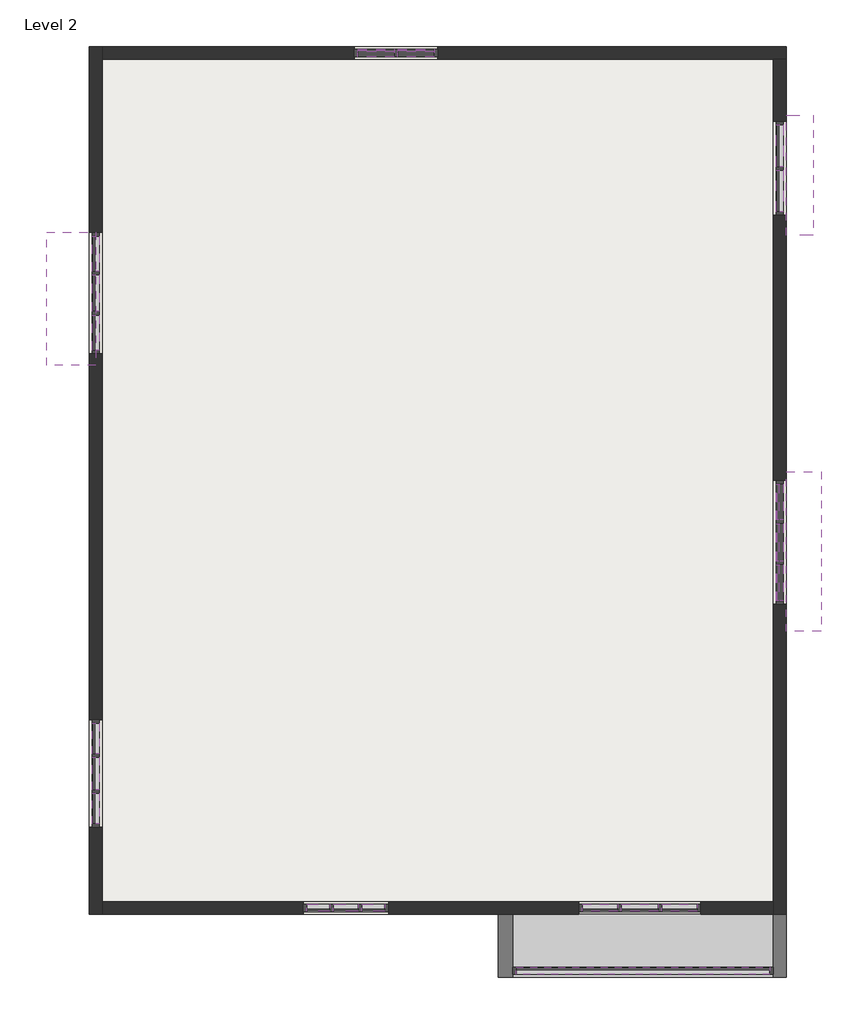
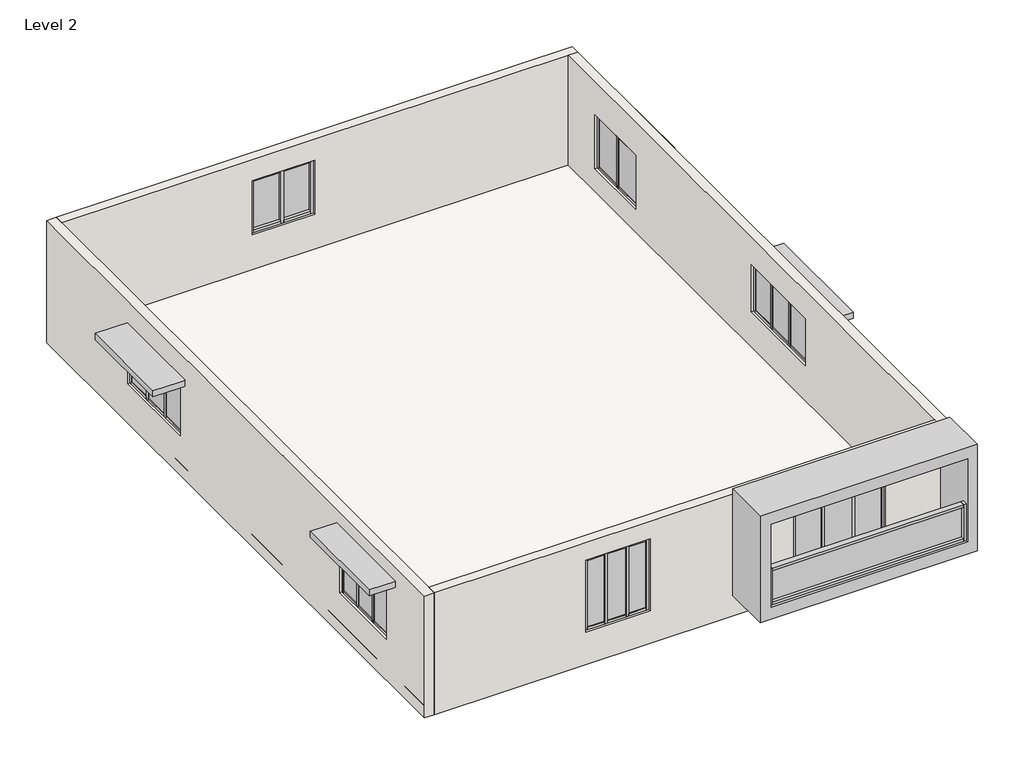
# One storey: 68 members, 20 plates, 4 proxies, 4 walls, 1 roof.
"""IFC4 building model written with IfcOpenShell, lengths in millimetres."""

from ifc_helpers import new_model, si_unit, frame, origin, place, context, project, spatial, polyline, outline, extrude, faceted_brep, transform, mapped, element, save
from components import generic_models_10_generic_models_10_e59920a7, generic_models_13_generic_models_13_81a3a1d9, generic_models_4_generic_models_4_7a9117e9, generic_models_9_generic_models_9_c0a8784b, member_bc7dbe04, member_dc106669, member_3fd415ec, member_f80a073c, member_00d99baf, member_d3852687, member_f51f5eff, member_1cdc6c9a, member_1d73318e, member_ea77439e, member_3a0a7659, member_051277f3, member_afffad75, member_dad99500, member_d9f78736, member_05f3a264, member_d4123ca4, member_668e8779, member_8c893cff, member_c9631cd1, member_eeb7212f, member_0bb20091, member_43a8b99b, member_a81ad59a, member_ef5723a8, member_5215b92c, member_553ffa17, member_c0163ebe, system_panel_glazed_42f26034, system_panel_glazed_4ea5c58e, system_panel_glazed_209adb3c, system_panel_glazed_df754354, system_panel_glazed_4996dcf2, system_panel_glazed_4f773535, system_panel_glazed_f0f913a6, system_panel_glazed_204414d1, system_panel_glazed_c810d226, system_panel_glazed_a6da17b0, system_panel_glazed_9e0010b7, system_panel_glazed_2a0e46e6, system_panel_glazed_327d625d

model = new_model("IFC4")

# Units and contexts
model_context = context("Model", 3, world=origin())
ifc_project = project(units=[si_unit("LENGTHUNIT", "METRE", prefix="MILLI")], contexts=[model_context])

# Site, building, storey
site = spatial("IfcSite", under=ifc_project)
building = spatial("IfcBuilding", under=site)
storey = spatial("IfcBuildingStorey", under=building, Name="Level 2", Elevation=3048.0)

# Proxies
placement = place(None, origin())
generic_models_10_generic_models_10_shape = generic_models_10_generic_models_10_e59920a7(model_context)
element("IfcBuildingElementProxy", 1, Name="Generic Models 10 : Generic Models 10", ObjectType="Generic Models 10 : Generic Models 10", at=placement, inside=storey, context=model_context, shape_type="MappedRepresentation", body=[
    mapped(generic_models_10_generic_models_10_shape, transform((0.0, 0.0, 0.0), x_axis=(1.0, 0.0, 0.0), y_axis=(0.0, 1.0, 0.0), z_axis=(0.0, 0.0, 1.0))),
])
generic_models_13_generic_models_13_shape = generic_models_13_generic_models_13_81a3a1d9(model_context)
element("IfcBuildingElementProxy", 2, Name="Generic Models 13 : Generic Models 13", ObjectType="Generic Models 13 : Generic Models 13", at=placement, inside=storey, context=model_context, shape_type="MappedRepresentation", body=[
    mapped(generic_models_13_generic_models_13_shape, transform((0.0, 0.0, 0.0), x_axis=(1.0, 0.0, 0.0), y_axis=(0.0, 1.0, 0.0), z_axis=(0.0, 0.0, 1.0))),
])
generic_models_4_generic_models_4_shape = generic_models_4_generic_models_4_7a9117e9(model_context)
element("IfcBuildingElementProxy", 3, Name="Generic Models 4 : Generic Models 4", ObjectType="Generic Models 4 : Generic Models 4", at=placement, inside=storey, context=model_context, shape_type="MappedRepresentation", body=[
    mapped(generic_models_4_generic_models_4_shape, transform((0.0, 0.0, 0.0), x_axis=(1.0, 0.0, 0.0), y_axis=(0.0, 1.0, 0.0), z_axis=(0.0, 0.0, 1.0))),
])
generic_models_9_generic_models_9_shape = generic_models_9_generic_models_9_c0a8784b(model_context)
element("IfcBuildingElementProxy", 4, Name="Generic Models 9 : Generic Models 9", ObjectType="Generic Models 9 : Generic Models 9", at=placement, inside=storey, context=model_context, shape_type="MappedRepresentation", body=[
    mapped(generic_models_9_generic_models_9_shape, transform((0.0, 0.0, 0.0), x_axis=(1.0, 0.0, 0.0), y_axis=(0.0, 1.0, 0.0), z_axis=(0.0, 0.0, 1.0))),
])

# Members
member_shape = member_bc7dbe04(model_context)
element("IfcMember", 5, ObjectType="Rectangular Mullion : 2.5\" x 5\" rectangular", at=placement, inside=storey, context=model_context, shape_type="MappedRepresentation", body=[
    mapped(member_shape, transform((-11428.8359258, -11686.7777232, 3860.2469154), x_axis=(0.0, 0.0, -1.0), y_axis=(0.0, 1.0, 0.0), z_axis=(1.0, 0.0, 0.0))),
])
member_2_shape = member_dc106669(model_context)
element("IfcMember", 6, ObjectType="Rectangular Mullion : 2.5\" x 5\" rectangular", at=placement, inside=storey, context=model_context, shape_type="MappedRepresentation", body=[
    mapped(member_2_shape, transform((-11936.8359258, -11686.7777232, 3860.2469154), x_axis=(0.0, 0.0, -1.0), y_axis=(0.0, 1.0, 0.0), z_axis=(1.0, 0.0, 0.0))),
])
element("IfcMember", 7, ObjectType="Rectangular Mullion : 2.5\" x 5\" rectangular", at=placement, inside=storey, context=model_context, shape_type="MappedRepresentation", body=[
    mapped(member_2_shape, transform((-10952.5859258, -11686.7777232, 3860.2469154), x_axis=(0.0, 0.0, -1.0), y_axis=(0.0, 1.0, 0.0), z_axis=(1.0, 0.0, 0.0))),
])
element("IfcMember", 8, ObjectType="Rectangular Mullion : 2.5\" x 5\" rectangular", at=placement, inside=storey, context=model_context, shape_type="MappedRepresentation", body=[
    mapped(member_2_shape, transform((-11365.3359258, -11686.7777232, 5656.7140305), x_axis=(0.0, 0.0, 1.0), y_axis=(0.0, 1.0, 0.0), z_axis=(-1.0, 0.0, 0.0))),
])
element("IfcMember", 9, ObjectType="Rectangular Mullion : 2.5\" x 5\" rectangular", at=placement, inside=storey, context=model_context, shape_type="MappedRepresentation", body=[
    mapped(member_2_shape, transform((-12349.5859258, -11686.7777232, 5656.7140305), x_axis=(0.0, 0.0, 1.0), y_axis=(0.0, 1.0, 0.0), z_axis=(-1.0, 0.0, 0.0))),
])
element("IfcMember", 10, ObjectType="Rectangular Mullion : 2.5\" x 5\" rectangular", at=placement, inside=storey, context=model_context, shape_type="MappedRepresentation", body=[
    mapped(member_shape, transform((-11873.3359258, -11686.7777232, 5656.7140305), x_axis=(0.0, 0.0, 1.0), y_axis=(0.0, 1.0, 0.0), z_axis=(-1.0, 0.0, 0.0))),
])
member_3_shape = member_3fd415ec(model_context)
element("IfcMember", 11, ObjectType="Rectangular Mullion : 2.5\" x 5\" rectangular", at=placement, inside=storey, context=model_context, shape_type="MappedRepresentation", body=[
    mapped(member_3_shape, transform((-11905.0859258, -11686.7777232, 3860.2469154), x_axis=(-1.0, 0.0, 0.0), y_axis=(0.0, 1.0, 0.0), z_axis=(0.0, 0.0, -1.0))),
])
element("IfcMember", 12, ObjectType="Rectangular Mullion : 2.5\" x 5\" rectangular", at=placement, inside=storey, context=model_context, shape_type="MappedRepresentation", body=[
    mapped(member_3_shape, transform((-11397.0859258, -11686.7777232, 3860.2469154), x_axis=(-1.0, 0.0, 0.0), y_axis=(0.0, 1.0, 0.0), z_axis=(0.0, 0.0, -1.0))),
])
member_4_shape = member_f80a073c(model_context)
element("IfcMember", 13, ObjectType="Rectangular Mullion : 2.5\" x 5\" rectangular", at=placement, inside=storey, context=model_context, shape_type="MappedRepresentation", body=[
    mapped(member_4_shape, transform((-12413.0859258, -11686.7777232, 3860.2469154), x_axis=(-1.0, 0.0, 0.0), y_axis=(0.0, 1.0, 0.0), z_axis=(0.0, 0.0, -1.0))),
])
element("IfcMember", 14, ObjectType="Rectangular Mullion : 2.5\" x 5\" rectangular", at=placement, inside=storey, context=model_context, shape_type="MappedRepresentation", body=[
    mapped(member_4_shape, transform((-10889.0859258, -11686.7777232, 5656.7140305), x_axis=(1.0, 0.0, 0.0), y_axis=(0.0, 1.0, 0.0), z_axis=(0.0, 0.0, 1.0))),
])
member_5_shape = member_00d99baf(model_context)
element("IfcMember", 15, ObjectType="Rectangular Mullion : 2.5\" x 5\" rectangular", at=placement, inside=storey, context=model_context, shape_type="MappedRepresentation", body=[
    mapped(member_5_shape, transform((-6018.6359258, -11686.7777232, 5933.9332237), x_axis=(0.0, 0.0, 1.0), y_axis=(0.0, 1.0, 0.0), z_axis=(-1.0, 0.0, 0.0))),
])
element("IfcMember", 16, ObjectType="Rectangular Mullion : 2.5\" x 5\" rectangular", at=placement, inside=storey, context=model_context, shape_type="MappedRepresentation", body=[
    mapped(member_5_shape, transform((-7434.6859258, -11686.7777232, 5933.9332237), x_axis=(0.0, 0.0, 1.0), y_axis=(0.0, 1.0, 0.0), z_axis=(-1.0, 0.0, 0.0))),
])
member_6_shape = member_d3852687(model_context)
element("IfcMember", 17, ObjectType="Rectangular Mullion : 2.5\" x 5\" rectangular", at=placement, inside=storey, context=model_context, shape_type="MappedRepresentation", body=[
    mapped(member_6_shape, transform((-6742.5359258, -11686.7777232, 5933.9332237), x_axis=(0.0, 0.0, 1.0), y_axis=(0.0, 1.0, 0.0), z_axis=(-1.0, 0.0, 0.0))),
])
element("IfcMember", 18, ObjectType="Rectangular Mullion : 2.5\" x 5\" rectangular", at=placement, inside=storey, context=model_context, shape_type="MappedRepresentation", body=[
    mapped(member_6_shape, transform((-6082.1359258, -11686.7777232, 3853.2485641), x_axis=(0.0, 0.0, -1.0), y_axis=(0.0, 1.0, 0.0), z_axis=(1.0, 0.0, 0.0))),
])
element("IfcMember", 19, ObjectType="Rectangular Mullion : 2.5\" x 5\" rectangular", at=placement, inside=storey, context=model_context, shape_type="MappedRepresentation", body=[
    mapped(member_5_shape, transform((-6806.0359258, -11686.7777232, 3853.2485641), x_axis=(0.0, 0.0, -1.0), y_axis=(0.0, 1.0, 0.0), z_axis=(1.0, 0.0, 0.0))),
])
element("IfcMember", 20, ObjectType="Rectangular Mullion : 2.5\" x 5\" rectangular", at=placement, inside=storey, context=model_context, shape_type="MappedRepresentation", body=[
    mapped(member_5_shape, transform((-5389.9859258, -11686.7777232, 3853.2485641), x_axis=(0.0, 0.0, -1.0), y_axis=(0.0, 1.0, 0.0), z_axis=(1.0, 0.0, 0.0))),
])
member_7_shape = member_f51f5eff(model_context)
element("IfcMember", 21, ObjectType="Rectangular Mullion : 2.5\" x 5\" rectangular", at=placement, inside=storey, context=model_context, shape_type="MappedRepresentation", body=[
    mapped(member_7_shape, transform((-6774.2859258, -11686.7777232, 3853.2485641), x_axis=(-1.0, 0.0, 0.0), y_axis=(0.0, 1.0, 0.0), z_axis=(0.0, 0.0, -1.0))),
])
element("IfcMember", 22, ObjectType="Rectangular Mullion : 2.5\" x 5\" rectangular", at=placement, inside=storey, context=model_context, shape_type="MappedRepresentation", body=[
    mapped(member_7_shape, transform((-6050.3859258, -11686.7777232, 3853.2485641), x_axis=(-1.0, 0.0, 0.0), y_axis=(0.0, 1.0, 0.0), z_axis=(0.0, 0.0, -1.0))),
])
member_8_shape = member_1cdc6c9a(model_context)
element("IfcMember", 23, ObjectType="Rectangular Mullion : 2.5\" x 5\" rectangular", at=placement, inside=storey, context=model_context, shape_type="MappedRepresentation", body=[
    mapped(member_8_shape, transform((-7498.1859258, -11686.7777232, 3853.2485641), x_axis=(-1.0, 0.0, 0.0), y_axis=(0.0, 1.0, 0.0), z_axis=(0.0, 0.0, -1.0))),
])
element("IfcMember", 24, ObjectType="Rectangular Mullion : 2.5\" x 5\" rectangular", at=placement, inside=storey, context=model_context, shape_type="MappedRepresentation", body=[
    mapped(member_8_shape, transform((-5326.4859258, -11686.7777232, 5933.9332237), x_axis=(1.0, 0.0, 0.0), y_axis=(0.0, 1.0, 0.0), z_axis=(0.0, 0.0, 1.0))),
])
member_9_shape = member_1d73318e(model_context)
element("IfcMember", 25, ObjectType="Rectangular Mullion : 2.5\" x 5\" rectangular", at=placement, inside=storey, context=model_context, shape_type="MappedRepresentation", body=[
    mapped(member_9_shape, transform((-8679.2859258, -12804.3777232, 4777.3649741), x_axis=(-1.0, 0.0, 0.0), y_axis=(0.0, -1.0, 0.0), z_axis=(0.0, 0.0, 1.0))),
])
member_10_shape = member_ea77439e(model_context)
element("IfcMember", 26, ObjectType="Rectangular Mullion : 2.5\" x 5\" rectangular", at=placement, inside=storey, context=model_context, shape_type="MappedRepresentation", body=[
    mapped(member_10_shape, transform((-4094.5859258, -12804.3777232, 4777.3649741), x_axis=(0.0, 0.0, 1.0), y_axis=(0.0, -1.0, 0.0), z_axis=(1.0, 0.0, 0.0))),
])
element("IfcMember", 27, ObjectType="Rectangular Mullion : 2.5\" x 5\" rectangular", at=placement, inside=storey, context=model_context, shape_type="MappedRepresentation", body=[
    mapped(member_10_shape, transform((-8615.7859258, -12804.3777232, 3860.2469154), x_axis=(0.0, 0.0, -1.0), y_axis=(0.0, -1.0, 0.0), z_axis=(-1.0, 0.0, 0.0))),
])
element("IfcMember", 28, ObjectType="Rectangular Mullion : 2.5\" x 5\" rectangular", at=placement, inside=storey, context=model_context, shape_type="MappedRepresentation", body=[
    mapped(member_9_shape, transform((-4031.0859258, -12804.3777232, 3860.2469154), x_axis=(1.0, 0.0, 0.0), y_axis=(0.0, -1.0, 0.0), z_axis=(0.0, 0.0, -1.0))),
])
member_11_shape = member_3a0a7659(model_context)
element("IfcMember", 29, ObjectType="Rectangular Mullion : 2.5\" x 5\" rectangular", at=placement, inside=storey, context=model_context, shape_type="MappedRepresentation", body=[
    mapped(member_11_shape, transform((-3916.7859258, 1527.5722768, 3931.1298826), x_axis=(0.0, 0.0, -1.0), y_axis=(1.0, 0.0, 0.0), z_axis=(0.0, -1.0, 0.0))),
])
element("IfcMember", 30, ObjectType="Rectangular Mullion : 2.5\" x 5\" rectangular", at=placement, inside=storey, context=model_context, shape_type="MappedRepresentation", body=[
    mapped(member_11_shape, transform((-3916.7859258, 721.1222768, 3931.1298826), x_axis=(0.0, 0.0, -1.0), y_axis=(1.0, 0.0, 0.0), z_axis=(0.0, -1.0, 0.0))),
])
element("IfcMember", 31, ObjectType="Rectangular Mullion : 2.5\" x 5\" rectangular", at=placement, inside=storey, context=model_context, shape_type="MappedRepresentation", body=[
    mapped(member_11_shape, transform((-3916.7859258, 1464.0722768, 5279.0460342), x_axis=(0.0, 0.0, 1.0), y_axis=(1.0, 0.0, 0.0), z_axis=(0.0, 1.0, 0.0))),
])
element("IfcMember", 32, ObjectType="Rectangular Mullion : 2.5\" x 5\" rectangular", at=placement, inside=storey, context=model_context, shape_type="MappedRepresentation", body=[
    mapped(member_11_shape, transform((-3916.7859258, 2270.5222768, 5279.0460342), x_axis=(0.0, 0.0, 1.0), y_axis=(1.0, 0.0, 0.0), z_axis=(0.0, 1.0, 0.0))),
])
member_12_shape = member_051277f3(model_context)
element("IfcMember", 33, ObjectType="Rectangular Mullion : 2.5\" x 5\" rectangular", at=placement, inside=storey, context=model_context, shape_type="MappedRepresentation", body=[
    mapped(member_12_shape, transform((-3916.7859258, -4835.1277232, 5410.2621354), x_axis=(0.0, 0.0, 1.0), y_axis=(1.0, 0.0, 0.0), z_axis=(0.0, 1.0, 0.0))),
])
member_13_shape = member_afffad75(model_context)
element("IfcMember", 34, ObjectType="Rectangular Mullion : 2.5\" x 5\" rectangular", at=placement, inside=storey, context=model_context, shape_type="MappedRepresentation", body=[
    mapped(member_13_shape, transform((-3916.7859258, -5539.9777232, 4236.0377626), x_axis=(0.0, 1.0, 0.0), y_axis=(1.0, 0.0, 0.0), z_axis=(0.0, 0.0, -1.0))),
])
element("IfcMember", 35, ObjectType="Rectangular Mullion : 2.5\" x 5\" rectangular", at=placement, inside=storey, context=model_context, shape_type="MappedRepresentation", body=[
    mapped(member_13_shape, transform((-3916.7859258, -4803.3777232, 4236.0377626), x_axis=(0.0, 1.0, 0.0), y_axis=(1.0, 0.0, 0.0), z_axis=(0.0, 0.0, -1.0))),
])
element("IfcMember", 36, ObjectType="Rectangular Mullion : 2.5\" x 5\" rectangular", at=placement, inside=storey, context=model_context, shape_type="MappedRepresentation", body=[
    mapped(member_12_shape, transform((-3916.7859258, -5508.2277232, 4236.0377626), x_axis=(0.0, 0.0, -1.0), y_axis=(1.0, 0.0, 0.0), z_axis=(0.0, -1.0, 0.0))),
])
member_14_shape = member_dad99500(model_context)
element("IfcMember", 37, ObjectType="Rectangular Mullion : 2.5\" x 5\" rectangular", at=placement, inside=storey, context=model_context, shape_type="MappedRepresentation", body=[
    mapped(member_14_shape, transform((-3916.7859258, -5571.7277232, 5410.2621354), x_axis=(0.0, 0.0, 1.0), y_axis=(1.0, 0.0, 0.0), z_axis=(0.0, 1.0, 0.0))),
])
element("IfcMember", 38, ObjectType="Rectangular Mullion : 2.5\" x 5\" rectangular", at=placement, inside=storey, context=model_context, shape_type="MappedRepresentation", body=[
    mapped(member_14_shape, transform((-3916.7859258, -4130.2777232, 5410.2621354), x_axis=(0.0, 0.0, 1.0), y_axis=(1.0, 0.0, 0.0), z_axis=(0.0, 1.0, 0.0))),
])
element("IfcMember", 39, ObjectType="Rectangular Mullion : 2.5\" x 5\" rectangular", at=placement, inside=storey, context=model_context, shape_type="MappedRepresentation", body=[
    mapped(member_14_shape, transform((-3916.7859258, -4771.6277232, 4236.0377626), x_axis=(0.0, 0.0, -1.0), y_axis=(1.0, 0.0, 0.0), z_axis=(0.0, -1.0, 0.0))),
])
element("IfcMember", 40, ObjectType="Rectangular Mullion : 2.5\" x 5\" rectangular", at=placement, inside=storey, context=model_context, shape_type="MappedRepresentation", body=[
    mapped(member_14_shape, transform((-3916.7859258, -6213.0777232, 4236.0377626), x_axis=(0.0, 0.0, -1.0), y_axis=(1.0, 0.0, 0.0), z_axis=(0.0, -1.0, 0.0))),
])
member_15_shape = member_d9f78736(model_context)
element("IfcMember", 41, ObjectType="Rectangular Mullion : 2.5\" x 5\" rectangular", at=placement, inside=storey, context=model_context, shape_type="MappedRepresentation", body=[
    mapped(member_15_shape, transform((-3916.7859258, -4066.7777232, 4236.0377626), x_axis=(0.0, 1.0, 0.0), y_axis=(1.0, 0.0, 0.0), z_axis=(0.0, 0.0, -1.0))),
])
element("IfcMember", 42, ObjectType="Rectangular Mullion : 2.5\" x 5\" rectangular", at=placement, inside=storey, context=model_context, shape_type="MappedRepresentation", body=[
    mapped(member_15_shape, transform((-3916.7859258, -6276.5777232, 5410.2621354), x_axis=(0.0, -1.0, 0.0), y_axis=(1.0, 0.0, 0.0), z_axis=(0.0, 0.0, 1.0))),
])
member_16_shape = member_05f3a264(model_context)
element("IfcMember", 43, ObjectType="Rectangular Mullion : 2.5\" x 5\" rectangular", at=placement, inside=storey, context=model_context, shape_type="MappedRepresentation", body=[
    mapped(member_16_shape, transform((-3916.7859258, 1495.8222768, 3931.1298826), x_axis=(0.0, 1.0, 0.0), y_axis=(1.0, 0.0, 0.0), z_axis=(0.0, 0.0, -1.0))),
])
member_17_shape = member_d4123ca4(model_context)
element("IfcMember", 44, ObjectType="Rectangular Mullion : 2.5\" x 5\" rectangular", at=placement, inside=storey, context=model_context, shape_type="MappedRepresentation", body=[
    mapped(member_17_shape, transform((-3916.7859258, 2334.0222768, 3931.1298826), x_axis=(0.0, 1.0, 0.0), y_axis=(1.0, 0.0, 0.0), z_axis=(0.0, 0.0, -1.0))),
])
element("IfcMember", 45, ObjectType="Rectangular Mullion : 2.5\" x 5\" rectangular", at=placement, inside=storey, context=model_context, shape_type="MappedRepresentation", body=[
    mapped(member_17_shape, transform((-3916.7859258, 657.6222768, 5279.0460342), x_axis=(0.0, -1.0, 0.0), y_axis=(1.0, 0.0, 0.0), z_axis=(0.0, 0.0, 1.0))),
])
member_18_shape = member_668e8779(model_context)
element("IfcMember", 46, ObjectType="Rectangular Mullion : 2.5\" x 5\" rectangular", at=placement, inside=storey, context=model_context, shape_type="MappedRepresentation", body=[
    mapped(member_18_shape, transform((-16108.7859258, -9641.2608351, 5598.9809912), x_axis=(0.0, 0.0, 1.0), y_axis=(1.0, 0.0, 0.0), z_axis=(0.0, 1.0, 0.0))),
])
element("IfcMember", 47, ObjectType="Rectangular Mullion : 2.5\" x 5\" rectangular", at=placement, inside=storey, context=model_context, shape_type="MappedRepresentation", body=[
    mapped(member_18_shape, transform((-16108.7859258, -8397.4777232, 5598.9809912), x_axis=(0.0, 0.0, 1.0), y_axis=(1.0, 0.0, 0.0), z_axis=(0.0, 1.0, 0.0))),
])
member_19_shape = member_8c893cff(model_context)
element("IfcMember", 48, ObjectType="Rectangular Mullion : 2.5\" x 5\" rectangular", at=placement, inside=storey, context=model_context, shape_type="MappedRepresentation", body=[
    mapped(member_19_shape, transform((-16108.7859258, -9003.4942792, 5598.9809912), x_axis=(0.0, 0.0, 1.0), y_axis=(1.0, 0.0, 0.0), z_axis=(0.0, 1.0, 0.0))),
])
member_20_shape = member_c9631cd1(model_context)
element("IfcMember", 49, ObjectType="Rectangular Mullion : 2.5\" x 5\" rectangular", at=placement, inside=storey, context=model_context, shape_type="MappedRepresentation", body=[
    mapped(member_20_shape, transform((-16108.7859258, -8971.7442792, 4077.0672739), x_axis=(0.0, 1.0, 0.0), y_axis=(1.0, 0.0, 0.0), z_axis=(0.0, 0.0, -1.0))),
])
element("IfcMember", 50, ObjectType="Rectangular Mullion : 2.5\" x 5\" rectangular", at=placement, inside=storey, context=model_context, shape_type="MappedRepresentation", body=[
    mapped(member_20_shape, transform((-16108.7859258, -9609.5108351, 4077.0672739), x_axis=(0.0, 1.0, 0.0), y_axis=(1.0, 0.0, 0.0), z_axis=(0.0, 0.0, -1.0))),
])
element("IfcMember", 51, ObjectType="Rectangular Mullion : 2.5\" x 5\" rectangular", at=placement, inside=storey, context=model_context, shape_type="MappedRepresentation", body=[
    mapped(member_19_shape, transform((-16108.7859258, -9577.7608351, 4077.0672739), x_axis=(0.0, 0.0, -1.0), y_axis=(1.0, 0.0, 0.0), z_axis=(0.0, -1.0, 0.0))),
])
element("IfcMember", 52, ObjectType="Rectangular Mullion : 2.5\" x 5\" rectangular", at=placement, inside=storey, context=model_context, shape_type="MappedRepresentation", body=[
    mapped(member_18_shape, transform((-16108.7859258, -8939.9942792, 4077.0672739), x_axis=(0.0, 0.0, -1.0), y_axis=(1.0, 0.0, 0.0), z_axis=(0.0, -1.0, 0.0))),
])
element("IfcMember", 53, ObjectType="Rectangular Mullion : 2.5\" x 5\" rectangular", at=placement, inside=storey, context=model_context, shape_type="MappedRepresentation", body=[
    mapped(member_18_shape, transform((-16108.7859258, -10183.7773911, 4077.0672739), x_axis=(0.0, 0.0, -1.0), y_axis=(1.0, 0.0, 0.0), z_axis=(0.0, -1.0, 0.0))),
])
member_21_shape = member_eeb7212f(model_context)
element("IfcMember", 54, ObjectType="Rectangular Mullion : 2.5\" x 5\" rectangular", at=placement, inside=storey, context=model_context, shape_type="MappedRepresentation", body=[
    mapped(member_21_shape, transform((-16108.7859258, -8333.9777232, 4077.0672739), x_axis=(0.0, 1.0, 0.0), y_axis=(1.0, 0.0, 0.0), z_axis=(0.0, 0.0, -1.0))),
])
element("IfcMember", 55, ObjectType="Rectangular Mullion : 2.5\" x 5\" rectangular", at=placement, inside=storey, context=model_context, shape_type="MappedRepresentation", body=[
    mapped(member_21_shape, transform((-16108.7859258, -10247.2773911, 5598.9809912), x_axis=(0.0, -1.0, 0.0), y_axis=(1.0, 0.0, 0.0), z_axis=(0.0, 0.0, 1.0))),
])
member_22_shape = member_0bb20091(model_context)
element("IfcMember", 56, ObjectType="Rectangular Mullion : 2.5\" x 5\" rectangular", at=placement, inside=storey, context=model_context, shape_type="MappedRepresentation", body=[
    mapped(member_22_shape, transform((-16108.7859258, -1117.9456793, 5399.696684), x_axis=(0.0, 0.0, 1.0), y_axis=(1.0, 0.0, 0.0), z_axis=(0.0, 1.0, 0.0))),
])
element("IfcMember", 57, ObjectType="Rectangular Mullion : 2.5\" x 5\" rectangular", at=placement, inside=storey, context=model_context, shape_type="MappedRepresentation", body=[
    mapped(member_22_shape, transform((-16108.7859258, 290.1460165, 5399.696684), x_axis=(0.0, 0.0, 1.0), y_axis=(1.0, 0.0, 0.0), z_axis=(0.0, 1.0, 0.0))),
])
member_23_shape = member_43a8b99b(model_context)
element("IfcMember", 58, ObjectType="Rectangular Mullion : 2.5\" x 5\" rectangular", at=placement, inside=storey, context=model_context, shape_type="MappedRepresentation", body=[
    mapped(member_23_shape, transform((-16108.7859258, -398.0248314, 5399.696684), x_axis=(0.0, 0.0, 1.0), y_axis=(1.0, 0.0, 0.0), z_axis=(0.0, 1.0, 0.0))),
])
member_24_shape = member_a81ad59a(model_context)
element("IfcMember", 59, ObjectType="Rectangular Mullion : 2.5\" x 5\" rectangular", at=placement, inside=storey, context=model_context, shape_type="MappedRepresentation", body=[
    mapped(member_24_shape, transform((-16108.7859258, -366.2748314, 4034.2356799), x_axis=(0.0, 1.0, 0.0), y_axis=(1.0, 0.0, 0.0), z_axis=(0.0, 0.0, -1.0))),
])
element("IfcMember", 60, ObjectType="Rectangular Mullion : 2.5\" x 5\" rectangular", at=placement, inside=storey, context=model_context, shape_type="MappedRepresentation", body=[
    mapped(member_24_shape, transform((-16108.7859258, -1086.1956793, 4034.2356799), x_axis=(0.0, 1.0, 0.0), y_axis=(1.0, 0.0, 0.0), z_axis=(0.0, 0.0, -1.0))),
])
element("IfcMember", 61, ObjectType="Rectangular Mullion : 2.5\" x 5\" rectangular", at=placement, inside=storey, context=model_context, shape_type="MappedRepresentation", body=[
    mapped(member_23_shape, transform((-16108.7859258, -1054.4456793, 4034.2356799), x_axis=(0.0, 0.0, -1.0), y_axis=(1.0, 0.0, 0.0), z_axis=(0.0, -1.0, 0.0))),
])
element("IfcMember", 62, ObjectType="Rectangular Mullion : 2.5\" x 5\" rectangular", at=placement, inside=storey, context=model_context, shape_type="MappedRepresentation", body=[
    mapped(member_22_shape, transform((-16108.7859258, -334.5248314, 4034.2356799), x_axis=(0.0, 0.0, -1.0), y_axis=(1.0, 0.0, 0.0), z_axis=(0.0, -1.0, 0.0))),
])
element("IfcMember", 63, ObjectType="Rectangular Mullion : 2.5\" x 5\" rectangular", at=placement, inside=storey, context=model_context, shape_type="MappedRepresentation", body=[
    mapped(member_22_shape, transform((-16108.7859258, -1742.6165273, 4034.2356799), x_axis=(0.0, 0.0, -1.0), y_axis=(1.0, 0.0, 0.0), z_axis=(0.0, -1.0, 0.0))),
])
member_25_shape = member_ef5723a8(model_context)
element("IfcMember", 64, ObjectType="Rectangular Mullion : 2.5\" x 5\" rectangular", at=placement, inside=storey, context=model_context, shape_type="MappedRepresentation", body=[
    mapped(member_25_shape, transform((-16108.7859258, 353.6460165, 4034.2356799), x_axis=(0.0, 1.0, 0.0), y_axis=(1.0, 0.0, 0.0), z_axis=(0.0, 0.0, -1.0))),
])
element("IfcMember", 65, ObjectType="Rectangular Mullion : 2.5\" x 5\" rectangular", at=placement, inside=storey, context=model_context, shape_type="MappedRepresentation", body=[
    mapped(member_25_shape, transform((-16108.7859258, -1806.1165273, 5399.696684), x_axis=(0.0, -1.0, 0.0), y_axis=(1.0, 0.0, 0.0), z_axis=(0.0, 0.0, 1.0))),
])
member_26_shape = member_5215b92c(model_context)
element("IfcMember", 66, ObjectType="Rectangular Mullion : 2.5\" x 5\" rectangular", at=placement, inside=storey, context=model_context, shape_type="MappedRepresentation", body=[
    mapped(member_26_shape, transform((-10787.4859258, 3553.2222768, 5569.8192996), x_axis=(0.0, 0.0, 1.0), y_axis=(0.0, -1.0, 0.0), z_axis=(1.0, 0.0, 0.0))),
])
element("IfcMember", 67, ObjectType="Rectangular Mullion : 2.5\" x 5\" rectangular", at=placement, inside=storey, context=model_context, shape_type="MappedRepresentation", body=[
    mapped(member_26_shape, transform((-10076.2859258, 3553.2222768, 5569.8192996), x_axis=(0.0, 0.0, 1.0), y_axis=(0.0, -1.0, 0.0), z_axis=(1.0, 0.0, 0.0))),
])
member_27_shape = member_553ffa17(model_context)
element("IfcMember", 68, ObjectType="Rectangular Mullion : 2.5\" x 5\" rectangular", at=placement, inside=storey, context=model_context, shape_type="MappedRepresentation", body=[
    mapped(member_27_shape, transform((-10755.7359258, 3553.2222768, 4220.8322833), x_axis=(1.0, 0.0, 0.0), y_axis=(0.0, -1.0, 0.0), z_axis=(0.0, 0.0, -1.0))),
])
element("IfcMember", 69, ObjectType="Rectangular Mullion : 2.5\" x 5\" rectangular", at=placement, inside=storey, context=model_context, shape_type="MappedRepresentation", body=[
    mapped(member_26_shape, transform((-10723.9859258, 3553.2222768, 4220.8322833), x_axis=(0.0, 0.0, -1.0), y_axis=(0.0, -1.0, 0.0), z_axis=(-1.0, 0.0, 0.0))),
])
element("IfcMember", 70, ObjectType="Rectangular Mullion : 2.5\" x 5\" rectangular", at=placement, inside=storey, context=model_context, shape_type="MappedRepresentation", body=[
    mapped(member_26_shape, transform((-11435.1859258, 3553.2222768, 4220.8322833), x_axis=(0.0, 0.0, -1.0), y_axis=(0.0, -1.0, 0.0), z_axis=(-1.0, 0.0, 0.0))),
])
member_28_shape = member_c0163ebe(model_context)
element("IfcMember", 71, ObjectType="Rectangular Mullion : 2.5\" x 5\" rectangular", at=placement, inside=storey, context=model_context, shape_type="MappedRepresentation", body=[
    mapped(member_28_shape, transform((-10012.7859258, 3553.2222768, 4220.8322833), x_axis=(1.0, 0.0, 0.0), y_axis=(0.0, -1.0, 0.0), z_axis=(0.0, 0.0, -1.0))),
])
element("IfcMember", 72, ObjectType="Rectangular Mullion : 2.5\" x 5\" rectangular", at=placement, inside=storey, context=model_context, shape_type="MappedRepresentation", body=[
    mapped(member_28_shape, transform((-11498.6859258, 3553.2222768, 5569.8192996), x_axis=(-1.0, 0.0, 0.0), y_axis=(0.0, -1.0, 0.0), z_axis=(0.0, 0.0, 1.0))),
])

# Plates
system_panel_glazed_shape = system_panel_glazed_42f26034(model_context)
element("IfcPlate", 73, ObjectType="System Panel : Glazed", at=placement, inside=storey, context=model_context, shape_type="MappedRepresentation", body=[
    mapped(system_panel_glazed_shape, transform((-11158.9609258, -11686.7777232, 3923.7469154), x_axis=(-1.0, 0.0, 0.0), y_axis=(0.0, -1.0, 0.0), z_axis=(0.0, 0.0, 1.0))),
])
element("IfcPlate", 74, ObjectType="System Panel : Glazed", at=placement, inside=storey, context=model_context, shape_type="MappedRepresentation", body=[
    mapped(system_panel_glazed_shape, transform((-12143.2109258, -11686.7777232, 3923.7469154), x_axis=(-1.0, 0.0, 0.0), y_axis=(0.0, -1.0, 0.0), z_axis=(0.0, 0.0, 1.0))),
])
system_panel_glazed_2_shape = system_panel_glazed_4ea5c58e(model_context)
element("IfcPlate", 75, ObjectType="System Panel : Glazed", at=placement, inside=storey, context=model_context, shape_type="MappedRepresentation", body=[
    mapped(system_panel_glazed_2_shape, transform((-11651.0859258, -11686.7777232, 3923.7469154), x_axis=(-1.0, 0.0, 0.0), y_axis=(0.0, -1.0, 0.0), z_axis=(0.0, 0.0, 1.0))),
])
system_panel_glazed_3_shape = system_panel_glazed_209adb3c(model_context)
element("IfcPlate", 76, ObjectType="System Panel : Glazed", at=placement, inside=storey, context=model_context, shape_type="MappedRepresentation", body=[
    mapped(system_panel_glazed_3_shape, transform((-5704.3109258, -11686.7777232, 3916.7485641), x_axis=(-1.0, 0.0, 0.0), y_axis=(0.0, -1.0, 0.0), z_axis=(0.0, 0.0, 1.0))),
])
element("IfcPlate", 77, ObjectType="System Panel : Glazed", at=placement, inside=storey, context=model_context, shape_type="MappedRepresentation", body=[
    mapped(system_panel_glazed_3_shape, transform((-7120.3609258, -11686.7777232, 3916.7485641), x_axis=(-1.0, 0.0, 0.0), y_axis=(0.0, -1.0, 0.0), z_axis=(0.0, 0.0, 1.0))),
])
system_panel_glazed_4_shape = system_panel_glazed_df754354(model_context)
element("IfcPlate", 78, ObjectType="System Panel : Glazed", at=placement, inside=storey, context=model_context, shape_type="MappedRepresentation", body=[
    mapped(system_panel_glazed_4_shape, transform((-6412.3359258, -11686.7777232, 3916.7485641), x_axis=(-1.0, 0.0, 0.0), y_axis=(0.0, -1.0, 0.0), z_axis=(0.0, 0.0, 1.0))),
])
system_panel_glazed_5_shape = system_panel_glazed_4996dcf2(model_context)
element("IfcPlate", 79, ObjectType="System Panel : Glazed", at=placement, inside=storey, context=model_context, shape_type="MappedRepresentation", body=[
    mapped(system_panel_glazed_5_shape, transform((-6355.1859258, -12804.3777232, 3923.7469154), x_axis=(1.0, 0.0, 0.0), y_axis=(0.0, 1.0, 0.0), z_axis=(0.0, 0.0, 1.0))),
])
system_panel_glazed_6_shape = system_panel_glazed_4f773535(model_context)
element("IfcPlate", 80, ObjectType="System Panel : Glazed", at=placement, inside=storey, context=model_context, shape_type="MappedRepresentation", body=[
    mapped(system_panel_glazed_6_shape, transform((-3916.7859258, -5171.6777232, 4299.5377626), x_axis=(0.0, 1.0, 0.0), y_axis=(-1.0, 0.0, 0.0), z_axis=(0.0, 0.0, 1.0))),
])
system_panel_glazed_7_shape = system_panel_glazed_f0f913a6(model_context)
element("IfcPlate", 81, ObjectType="System Panel : Glazed", at=placement, inside=storey, context=model_context, shape_type="MappedRepresentation", body=[
    mapped(system_panel_glazed_7_shape, transform((-3916.7859258, -5892.4027232, 4299.5377626), x_axis=(0.0, 1.0, 0.0), y_axis=(-1.0, 0.0, 0.0), z_axis=(0.0, 0.0, 1.0))),
])
element("IfcPlate", 82, ObjectType="System Panel : Glazed", at=placement, inside=storey, context=model_context, shape_type="MappedRepresentation", body=[
    mapped(system_panel_glazed_7_shape, transform((-3916.7859258, -4450.9527232, 4299.5377626), x_axis=(0.0, 1.0, 0.0), y_axis=(-1.0, 0.0, 0.0), z_axis=(0.0, 0.0, 1.0))),
])
system_panel_glazed_8_shape = system_panel_glazed_204414d1(model_context)
element("IfcPlate", 83, ObjectType="System Panel : Glazed", at=placement, inside=storey, context=model_context, shape_type="MappedRepresentation", body=[
    mapped(system_panel_glazed_8_shape, transform((-3916.7859258, 1092.5972768, 3994.6298826), x_axis=(0.0, 1.0, 0.0), y_axis=(-1.0, 0.0, 0.0), z_axis=(0.0, 0.0, 1.0))),
])
element("IfcPlate", 84, ObjectType="System Panel : Glazed", at=placement, inside=storey, context=model_context, shape_type="MappedRepresentation", body=[
    mapped(system_panel_glazed_8_shape, transform((-3916.7859258, 1899.0472768, 3994.6298826), x_axis=(0.0, 1.0, 0.0), y_axis=(-1.0, 0.0, 0.0), z_axis=(0.0, 0.0, 1.0))),
])
system_panel_glazed_9_shape = system_panel_glazed_c810d226(model_context)
element("IfcPlate", 85, ObjectType="System Panel : Glazed", at=placement, inside=storey, context=model_context, shape_type="MappedRepresentation", body=[
    mapped(system_panel_glazed_9_shape, transform((-16108.7859258, -9912.5191131, 4140.5672739), x_axis=(0.0, 1.0, 0.0), y_axis=(-1.0, 0.0, 0.0), z_axis=(0.0, 0.0, 1.0))),
])
element("IfcPlate", 86, ObjectType="System Panel : Glazed", at=placement, inside=storey, context=model_context, shape_type="MappedRepresentation", body=[
    mapped(system_panel_glazed_9_shape, transform((-16108.7859258, -8668.7360012, 4140.5672739), x_axis=(0.0, 1.0, 0.0), y_axis=(-1.0, 0.0, 0.0), z_axis=(0.0, 0.0, 1.0))),
])
system_panel_glazed_10_shape = system_panel_glazed_a6da17b0(model_context)
element("IfcPlate", 87, ObjectType="System Panel : Glazed", at=placement, inside=storey, context=model_context, shape_type="MappedRepresentation", body=[
    mapped(system_panel_glazed_10_shape, transform((-16108.7859258, -9290.6275571, 4140.5672739), x_axis=(0.0, 1.0, 0.0), y_axis=(-1.0, 0.0, 0.0), z_axis=(0.0, 0.0, 1.0))),
])
system_panel_glazed_11_shape = system_panel_glazed_9e0010b7(model_context)
element("IfcPlate", 88, ObjectType="System Panel : Glazed", at=placement, inside=storey, context=model_context, shape_type="MappedRepresentation", body=[
    mapped(system_panel_glazed_11_shape, transform((-16108.7859258, -1430.2811033, 4097.7356799), x_axis=(0.0, 1.0, 0.0), y_axis=(-1.0, 0.0, 0.0), z_axis=(0.0, 0.0, 1.0))),
])
element("IfcPlate", 89, ObjectType="System Panel : Glazed", at=placement, inside=storey, context=model_context, shape_type="MappedRepresentation", body=[
    mapped(system_panel_glazed_11_shape, transform((-16108.7859258, -22.1894074, 4097.7356799), x_axis=(0.0, 1.0, 0.0), y_axis=(-1.0, 0.0, 0.0), z_axis=(0.0, 0.0, 1.0))),
])
system_panel_glazed_12_shape = system_panel_glazed_2a0e46e6(model_context)
element("IfcPlate", 90, ObjectType="System Panel : Glazed", at=placement, inside=storey, context=model_context, shape_type="MappedRepresentation", body=[
    mapped(system_panel_glazed_12_shape, transform((-16108.7859258, -726.2352554, 4097.7356799), x_axis=(0.0, 1.0, 0.0), y_axis=(-1.0, 0.0, 0.0), z_axis=(0.0, 0.0, 1.0))),
])
system_panel_glazed_13_shape = system_panel_glazed_327d625d(model_context)
element("IfcPlate", 91, ObjectType="System Panel : Glazed", at=placement, inside=storey, context=model_context, shape_type="MappedRepresentation", body=[
    mapped(system_panel_glazed_13_shape, transform((-11111.3359258, 3553.2222768, 4284.3322833), x_axis=(1.0, 0.0, 0.0), y_axis=(0.0, 1.0, 0.0), z_axis=(0.0, 0.0, 1.0))),
])
element("IfcPlate", 92, ObjectType="System Panel : Glazed", at=placement, inside=storey, context=model_context, shape_type="MappedRepresentation", body=[
    mapped(system_panel_glazed_13_shape, transform((-10400.1359258, 3553.2222768, 4284.3322833), x_axis=(1.0, 0.0, 0.0), y_axis=(0.0, 1.0, 0.0), z_axis=(0.0, 0.0, 1.0))),
])

# Roof
element("IfcRoof", 93, ObjectType="Generic - 12\"", at=placement, inside=storey, context=model_context, shape_type="SweptSolid", body=[
    extrude(outline(polyline([(-16223.0859258, 3667.5222768), (-3802.4859258, 3667.5222768), (-3802.4859258, -11801.0777232), (-16223.0859258, -11801.0777232), (-16223.0859258, 3667.5222768)])), frame((0.0, 0.0, 3048.0), z_axis=(0.0, 0.0, 1.0), x_axis=(1.0, 0.0, 0.0)), (0.0, 0.0, 1.0), 304.8),
])

# Walls
element("IfcWall", 94, ObjectType="9\"", at=placement, inside=storey, context=model_context, shape_type="Brep", body=[
    faceted_brep([(-15994.4859258, -11801.0777232, 3048.0), (-15994.4859258, -11572.4777232, 3048.0), (-15994.4859258, 3438.9222768, 3048.0), (-15994.4859258, 3667.5222768, 3048.0), (-15994.4859258, 3667.5222768, 6096.0), (-15994.4859258, 3438.9222768, 6096.0), (-15994.4859258, -11572.4777232, 6096.0), (-15994.4859258, -11801.0777232, 6096.0), (-15994.4859258, -10247.2773911, 4077.0672739), (-15994.4859258, -10247.2773911, 5598.9809912), (-15994.4859258, -8333.9777232, 5598.9809912), (-15994.4859258, -8333.9777232, 4077.0672739), (-15994.4859258, -1806.1165273, 4034.2356799), (-15994.4859258, -1806.1165273, 5399.696684), (-15994.4859258, 353.6460165, 5399.696684), (-15994.4859258, 353.6460165, 4034.2356799), (-16223.0859258, 3667.5222768, 3048.0), (-16223.0859258, -11801.0777232, 3048.0), (-16223.0859258, -11801.0777232, 6096.0), (-16223.0859258, 3667.5222768, 6096.0), (-16223.0859258, -10247.2773911, 5598.9809912), (-16223.0859258, -10247.2773911, 4077.0672739), (-16223.0859258, -8333.9777232, 4077.0672739), (-16223.0859258, -8333.9777232, 5598.9809912), (-16223.0859258, -1806.1165273, 5399.696684), (-16223.0859258, -1806.1165273, 4034.2356799), (-16223.0859258, 353.6460165, 4034.2356799), (-16223.0859258, 353.6460165, 5399.696684)], [[[0, 1, 2, 3, 4, 5, 6, 7], [8, 9, 10, 11], [12, 13, 14, 15]], [[16, 17, 18, 19], [20, 21, 22, 23], [24, 25, 26, 27]], [[3, 2, 1, 0, 17, 16]], [[7, 6, 5, 4, 19, 18]], [[4, 3, 16, 19]], [[0, 7, 18, 17]], [[8, 21, 20, 9]], [[9, 20, 23, 10]], [[10, 23, 22, 11]], [[21, 8, 11, 22]], [[12, 25, 24, 13]], [[13, 24, 27, 14]], [[26, 15, 14, 27]], [[25, 12, 15, 26]]]),
])
element("IfcWall", 95, ObjectType="9\"", at=placement, inside=storey, context=model_context, shape_type="Brep", body=[
    faceted_brep([(-15994.4859258, 3438.9222768, 3048.0), (-4031.0859258, 3438.9222768, 3048.0), (-3802.4859258, 3438.9222768, 3048.0), (-3802.4859258, 3438.9222768, 6096.0), (-4031.0859258, 3438.9222768, 6096.0), (-15994.4859258, 3438.9222768, 6096.0), (-11498.6859258, 3438.9222768, 4220.8322833), (-11498.6859258, 3438.9222768, 5569.8192996), (-10012.7859258, 3438.9222768, 5569.8192996), (-10012.7859258, 3438.9222768, 4220.8322833), (-3802.4859258, 3667.5222768, 3048.0), (-15994.4859258, 3667.5222768, 3048.0), (-15994.4859258, 3667.5222768, 6096.0), (-3802.4859258, 3667.5222768, 6096.0), (-11498.6859258, 3667.5222768, 5569.8192996), (-11498.6859258, 3667.5222768, 4220.8322833), (-10012.7859258, 3667.5222768, 4220.8322833), (-10012.7859258, 3667.5222768, 5569.8192996)], [[[0, 1, 2, 3, 4, 5], [6, 7, 8, 9]], [[10, 11, 12, 13], [14, 15, 16, 17]], [[2, 1, 0, 11, 10]], [[5, 4, 3, 13, 12]], [[0, 5, 12, 11]], [[3, 2, 10, 13]], [[6, 15, 14, 7]], [[7, 14, 17, 8]], [[8, 17, 16, 9]], [[15, 6, 9, 16]]]),
])
element("IfcWall", 96, ObjectType="9\"", at=placement, inside=storey, context=model_context, shape_type="Brep", body=[
    faceted_brep([(-4031.0859258, 3438.9222768, 3048.0), (-4031.0859258, -11572.4777232, 3048.0), (-4031.0859258, -11801.0777232, 3048.0), (-4031.0859258, -11801.0777232, 6096.0), (-4031.0859258, -11572.4777232, 6096.0), (-4031.0859258, 3438.9222768, 6096.0), (-4031.0859258, -6276.5777232, 5410.2621354), (-4031.0859258, -6276.5777232, 4236.0377626), (-4031.0859258, -4066.7777232, 4236.0377626), (-4031.0859258, -4066.7777232, 5410.2621354), (-4031.0859258, 657.6222768, 5279.0460342), (-4031.0859258, 657.6222768, 3931.1298826), (-4031.0859258, 2334.0222768, 3931.1298826), (-4031.0859258, 2334.0222768, 5279.0460342), (-3802.4859258, -11801.0777232, 3048.0), (-3802.4859258, 3438.9222768, 3048.0), (-3802.4859258, 3438.9222768, 6096.0), (-3802.4859258, -11801.0777232, 6096.0), (-3802.4859258, -6276.5777232, 4236.0377626), (-3802.4859258, -6276.5777232, 5410.2621354), (-3802.4859258, -4066.7777232, 5410.2621354), (-3802.4859258, -4066.7777232, 4236.0377626), (-3802.4859258, 657.6222768, 3931.1298826), (-3802.4859258, 657.6222768, 5279.0460342), (-3802.4859258, 2334.0222768, 5279.0460342), (-3802.4859258, 2334.0222768, 3931.1298826)], [[[0, 1, 2, 3, 4, 5], [6, 7, 8, 9], [10, 11, 12, 13]], [[14, 15, 16, 17], [18, 19, 20, 21], [22, 23, 24, 25]], [[2, 1, 0, 15, 14]], [[5, 4, 3, 17, 16]], [[0, 5, 16, 15]], [[3, 2, 14, 17]], [[18, 7, 6, 19]], [[19, 6, 9, 20]], [[20, 9, 8, 21]], [[7, 18, 21, 8]], [[22, 11, 10, 23]], [[23, 10, 13, 24]], [[12, 25, 24, 13]], [[11, 22, 25, 12]]]),
])
element("IfcWall", 97, ObjectType="9\"", at=placement, inside=storey, context=model_context, shape_type="SweptSolid", body=[
    extrude(outline(polyline([(3048.0, -15994.4859258), (3048.0, -4031.0859258), (6096.0, -4031.0859258), (6096.0, -15994.4859258), (3048.0, -15994.4859258)]), holes=[polyline([(5933.9332237, -5326.4859258), (3853.2485641, -5326.4859258), (3853.2485641, -7498.1859258), (5933.9332237, -7498.1859258), (5933.9332237, -5326.4859258)]), polyline([(5656.7140305, -10889.0859258), (3860.2469154, -10889.0859258), (3860.2469154, -12413.0859258), (5656.7140305, -12413.0859258), (5656.7140305, -10889.0859258)])]), frame((0.0, -11801.0777232, 0.0), z_axis=(0.0, 1.0, 0.0), x_axis=(0.0, 0.0, 1.0)), (0.0, 0.0, 1.0), 228.6),
])

save(model, "model.ifc")

# Revit data of these elements
# Type "Rectangular Mullion : 2.5\" x 5\" rectangular"
#   built-in parameter 1007304 = 0.416667 (stored number, unit not read)
#   built-in parameter 1007301 = 0.104167 (stored number, unit not read)
#   built-in parameter 1007300 = 0.104167 (stored number, unit not read)
# Type "System Panel : Glazed"
#   Construction Type Id = "GSP4R"
#   Analytic Construction = "1/8 in Pilkington single glazing"
#   Visual Light Transmittance = 0.9
#   Solar Heat Gain Coefficient = 0.86
#   Heat Transfer Coefficient (U) = 1.18115 BTU/(h·ft²·°F)
#   Define Thermal Properties by = 1
# Type "Generic - 12\""
#   Assembly Code = "B1020"
#   Layers, outside or top first: 1' - 0" no material (function 1)
# Type "9\""
#   Assembly Code = "B2010"
#   Layers, outside or top first: 0' - 9" no material (function 1)
# Element 1 (IfcBuildingElementProxy, "Generic Models 10 : Generic Models 10")
#   Phase Created = New Construction
# Element 2 (IfcBuildingElementProxy, "Generic Models 13 : Generic Models 13")
#   Phase Created = New Construction
# Element 3 (IfcBuildingElementProxy, "Generic Models 4 : Generic Models 4")
#   Phase Created = New Construction
# Element 4 (IfcBuildingElementProxy, "Generic Models 9 : Generic Models 9")
#   Phase Created = New Construction
# Elements 5, 6, 7, 8, 9, 10, 11, 12, 13, 14, 15, 16, 17, 18, 19, 20, 21, 22, 23, 24, 25, 26, 27, 28, 29, 30, 31, 32, 33, 34, 35, 36, 37, 38, 39, 40, 41, 42, 43, 44, 45, 46, 47, 48, 49, 50, 51, 52, 53, 54, 55, 56, 57, 58, 59, 60, 61, 62, 63, 64, 65, 66, 67, 68, 69, 70, 71, 72 (IfcMember, "Rectangular Mullion : 2.5\" x 5\" rectangular")
#   Phase Created = New Construction
#   Materials on its faces: "Aluminum"
# Elements 73, 74, 75, 76, 77, 78, 79, 80, 81, 82, 83, 84, 85, 86, 87, 88, 89, 90, 91, 92 (IfcPlate, "System Panel : Glazed")
#   Phase Created = New Construction
#   Materials on its faces: "Glass"
# Element 93 (IfcRoof, "Generic - 12\"")
#   built-in parameter 1001705 = 11 (stored number, unit not read)
#   built-in parameter 1001710 = 33615
#   Phase Created = New Construction
#   Materials on its faces: "Default Roof"
# Elements 94, 95, 96, 97 (IfcWall, "9\"")
#   Top Offset = 0' - 0"
#   Base Offset = 0' - 0"
#   Unconnected Height = 10' - 0"
#   wall height = 10' - 0"
#   Phase Created = New Construction
#   Base Constraint = Level 2
#   Materials on its faces: "Default Wall"
# Materials
#   "Aluminum": class "Metal", colour RGB 247 247 247, transparency 0, Description = "Aluminum 6061", Cost = 0
#   "Glass": class "Glass", colour RGB 0 128 192, transparency 0.75, Description = "Soda Lime Glass", Cost = 0
#   "Default Roof": colour RGB 88 101 114, transparency 0, Cost = 0
#   "Default Wall": colour RGB 128 128 128, transparency 0, Cost = 0
